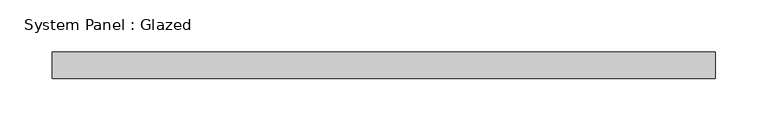
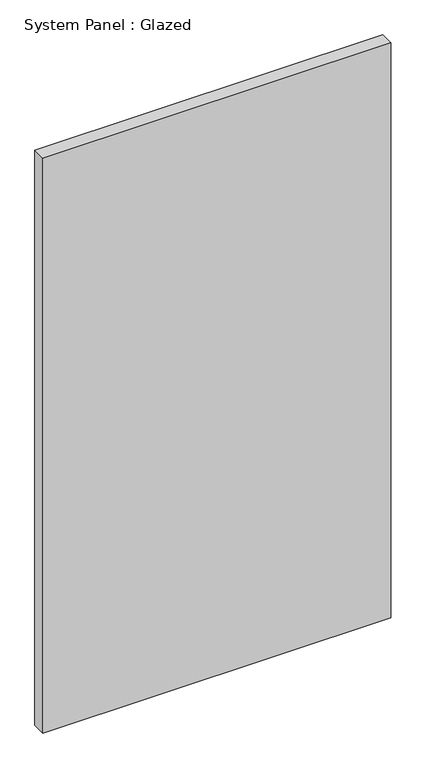
"""IFC4 building model written with IfcOpenShell, lengths in millimetres: plate geometry, System Panel : Glazed."""

from ifc_helpers import new_model, si_unit, origin, origin_with_axes, place, context, project, spatial, polyline, outline, extrude, source, transform, mapped, element, save


def system_panel_glazed_5a872b22(model_context):
    return source(origin(), model_context, "Body", "SweptSolid", [
        extrude(outline(polyline([(317.5, 19.05), (-317.5, 19.05), (-317.5, 44.45), (317.5, 44.45), (317.5, 19.05)])), origin_with_axes(), (0.0, 0.0, 1.0), 1109.7434076),
    ])


if __name__ == "__main__":
    model = new_model("IFC4")
    model_context = context("Model", 3, world=origin())
    ifc_project = project(units=[si_unit("LENGTHUNIT", "METRE", prefix="MILLI")], contexts=[model_context])
    site = spatial("IfcSite", under=ifc_project)
    building = spatial("IfcBuilding", under=site)
    placement = place(None, origin())
    system_panel_glazed_shape = system_panel_glazed_5a872b22(model_context)
    element("IfcPlate", 1, ObjectType="System Panel : Glazed", at=placement, inside=building, context=model_context, shape_type="MappedRepresentation", body=[
        mapped(system_panel_glazed_shape, transform((0.0, 0.0, 0.0), x_axis=(1.0, 0.0, 0.0), y_axis=(0.0, 1.0, 0.0), z_axis=(0.0, 0.0, 1.0))),
    ])
    save(model, "model.ifc")

# Revit data of these elements
# Type "System Panel : Glazed"
#   Construction Type Id = "GSP4R"
#   Analytic Construction = "1/8 in Pilkington single glazing"
#   Visual Light Transmittance = 0.9
#   Solar Heat Gain Coefficient = 0.86
#   Heat Transfer Coefficient (U) = 1.18115 BTU/(h·ft²·°F)
#   Define Thermal Properties by = 1
# Element 1 (IfcPlate, "System Panel : Glazed")
#   Materials on its faces: "Glass"
# Materials
#   "Glass": class "Glass", colour RGB 0 128 192, transparency 0.75, Description = "Soda Lime Glass", Cost = 0
